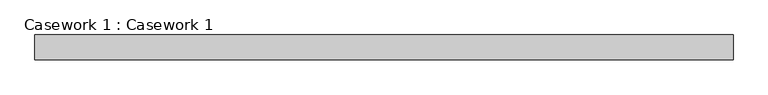
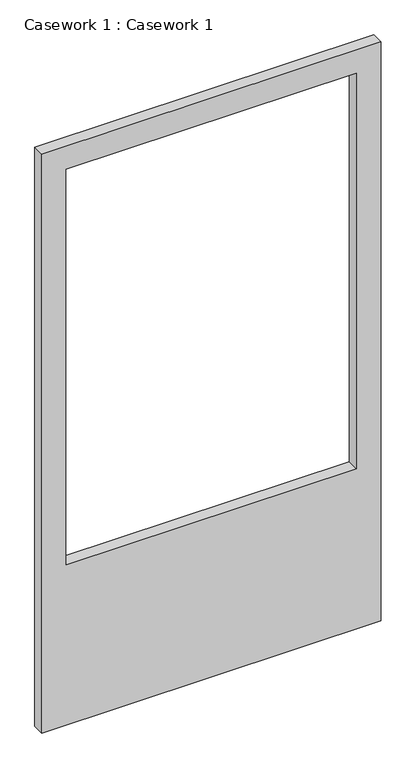
"""IFC4 building model written with IfcOpenShell, lengths in millimetres: furniture geometry, Casework 1 : Casework 1."""

from ifc_helpers import new_model, si_unit, frame, origin, place, context, project, spatial, polyline, outline, extrude, source, transform, mapped, element, save


def casework_1_casework_1_6c4e18a6(model_context):
    return source(origin(), model_context, "Body", "SweptSolid", [
        extrude(outline(polyline([(3797.4, -15472.8520625), (3797.4, -17577.6520625), (0.1, -17577.6520625), (0.1, -15472.8520625), (3797.4, -15472.8520625)]), holes=[polyline([(3645.0, -15625.2520625), (1050.0, -15625.2520625), (1050.0, -17425.2520625), (3645.0, -17425.2520625), (3645.0, -15625.2520625)])]), frame((0.0, -10301.0480844, 0.0), z_axis=(0.0, 1.0, 0.0), x_axis=(0.0, 0.0, 1.0)), (0.0, 0.0, 1.0), 75.0),
    ])


if __name__ == "__main__":
    model = new_model("IFC4")
    model_context = context("Model", 3, world=origin())
    ifc_project = project(units=[si_unit("LENGTHUNIT", "METRE", prefix="MILLI")], contexts=[model_context])
    site = spatial("IfcSite", under=ifc_project)
    building = spatial("IfcBuilding", under=site)
    placement = place(None, origin())
    casework_1_casework_1_shape = casework_1_casework_1_6c4e18a6(model_context)
    element("IfcFurniture", 1, ObjectType="Casework 1 : Casework 1", at=placement, inside=building, context=model_context, shape_type="MappedRepresentation", body=[
        mapped(casework_1_casework_1_shape, transform((0.0, 0.0, 0.0), x_axis=(1.0, 0.0, 0.0), y_axis=(0.0, 1.0, 0.0), z_axis=(0.0, 0.0, 1.0))),
    ])
    save(model, "model.ifc")
